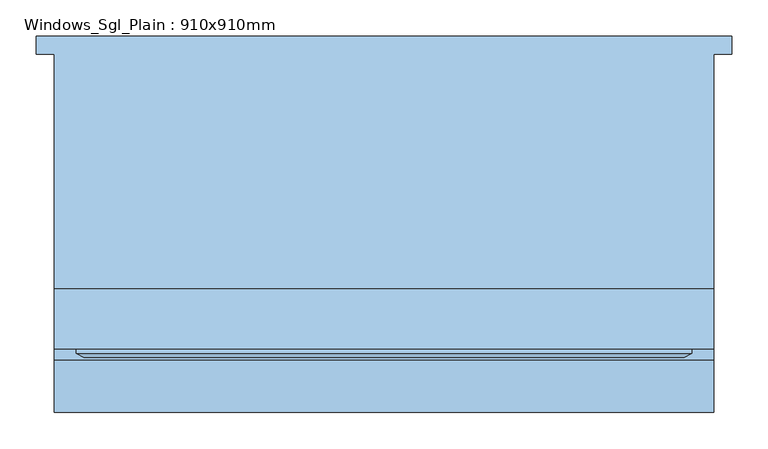
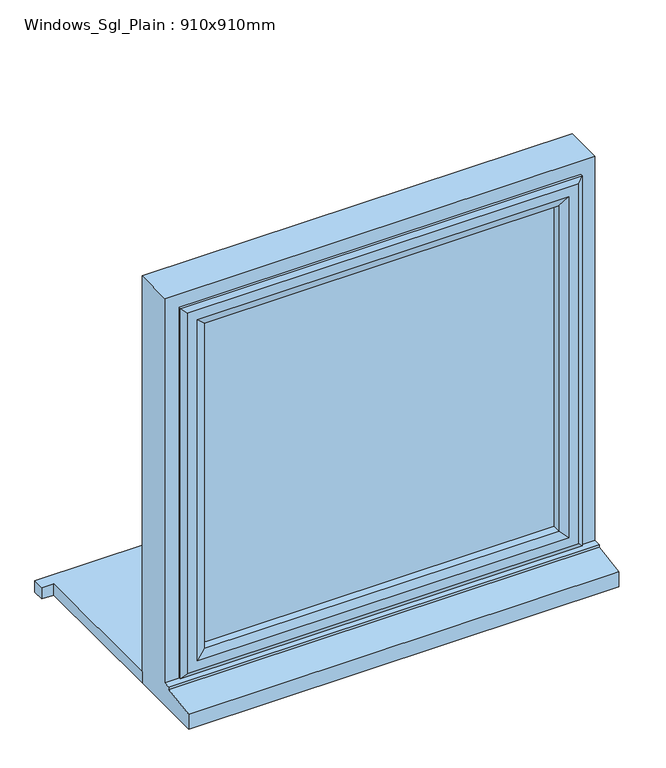
"""IFC4 building model written with IfcOpenShell, lengths in millimetres: window geometry, Windows_Sgl_Plain : 910x910mm."""

from ifc_helpers import new_model, si_unit, frame, origin, place, context, project, spatial, polyline, outline, extrude, faceted_brep, source, transform, mapped, element, save


def windows_sgl_plain_910x910mm_27dc79fa(model_context):
    return source(origin(), model_context, "Body", "SolidModel", [
        extrude(outline(polyline([(-480.0, 245.1434322), (480.0, 245.1434322), (480.0, 220.1434322), (455.0, 220.1434322), (455.0, -104.0565678), (-455.0, -104.0565678), (-455.0, 220.1434322), (-480.0, 220.1434322), (-480.0, 245.1434322)])), frame((0.0, 0.0, 1200.0), z_axis=(0.0, 0.0, 1.0), x_axis=(1.0, 0.0, 0.0)), (0.0, 0.0, 1.0), 25.0),
        faceted_brep([(-455.0, -104.0565678, 1200.0), (-455.0, -104.0565678, 2110.0), (455.0, -104.0565678, 2110.0), (455.0, -104.0565678, 1200.0), (-395.0, -104.0565678, 2050.0), (-395.0, -104.0565678, 1275.0), (395.0, -104.0565678, 1275.0), (395.0, -104.0565678, 2050.0), (-455.0, -274.5565678, 1200.0), (-455.0, -274.5565678, 1233.8088847), (-455.0, -202.0565678, 1244.7449676), (-455.0, -202.0565678, 1249.68767), (-455.0, -187.0565678, 1251.0), (-455.0, -187.0565678, 2110.0), (455.0, -187.0565678, 1251.0), (455.0, -187.0565678, 2110.0), (-415.0, -187.0565678, 2070.0), (415.0, -187.0565678, 2070.0), (415.0, -187.0565678, 1263.0), (-415.0, -187.0565678, 1263.0), (-415.0, -122.0565678, 1263.0), (-415.0, -122.0565678, 2070.0), (415.0, -122.0565678, 1263.0), (415.0, -122.0565678, 2070.0), (-395.0, -122.0565678, 2050.0), (395.0, -122.0565678, 2050.0), (395.0, -122.0565678, 1275.0), (-395.0, -122.0565678, 1275.0), (455.0, -202.0565678, 1249.68767), (455.0, -202.0565678, 1244.7449676), (455.0, -274.5565678, 1233.8088847), (455.0, -274.5565678, 1200.0)], [[[0, 1, 2, 3], [4, 5, 6, 7]], [[0, 8, 9, 10, 11, 12, 13, 1]], [[12, 14, 15, 13], [16, 17, 18, 19]], [[19, 20, 21, 16]], [[21, 20, 22, 23], [24, 25, 26, 27]], [[24, 27, 5, 4]], [[1, 13, 15, 2]], [[16, 21, 23, 17]], [[7, 25, 24, 4]], [[14, 28, 29, 30, 31, 3, 2, 15]], [[17, 23, 22, 18]], [[7, 6, 26, 25]], [[31, 8, 0, 3]], [[30, 9, 8, 31]], [[29, 10, 9, 30]], [[28, 11, 10, 29]], [[14, 12, 11, 28]], [[20, 19, 18, 22]], [[5, 27, 26, 6]]]),
        extrude(outline(polyline([(385.0, -151.0565678), (385.0, -175.0565678), (-385.0, -175.0565678), (-385.0, -151.0565678), (385.0, -151.0565678)])), frame((0.0, 0.0, 1293.0), z_axis=(0.0, 0.0, 1.0), x_axis=(1.0, 0.0, 0.0)), (0.0, 0.0, 1.0), 747.0),
        faceted_brep([(-425.0, -187.0565678, 2080.0), (-425.0, -187.0565678, 1253.0), (-425.0, -192.8300705, 1253.0), (-425.0, -192.8300705, 2080.0), (-415.0, -122.0565678, 2070.0), (-415.0, -122.0565678, 1263.0), (-415.0, -187.0565678, 1263.0), (-415.0, -187.0565678, 2070.0), (-375.0, -136.5494677, 2030.0), (-375.0, -136.5494677, 1303.0), (-385.1480377, -122.0565678, 1292.8519623), (-385.1480377, -122.0565678, 2040.1480377), (-375.0, -151.0565678, 2030.0), (-375.0, -151.0565678, 1303.0), (-385.0, -175.0565678, 2040.0), (-385.0, -175.0565678, 1293.0), (-385.0, -151.0565678, 1293.0), (-385.0, -151.0565678, 2040.0), (-375.0, -192.8300705, 2030.0), (-375.0, -192.8300705, 1303.0), (-375.0, -175.0565678, 1303.0), (-375.0, -175.0565678, 2030.0), (-392.4457548, -198.6035732, 2047.4457548), (-392.4457548, -198.6035732, 1285.5542452), (-414.2153903, -198.6035732, 1263.7846097), (-414.2153903, -198.6035732, 2069.2153903), (425.0, -187.0565678, 1253.0), (425.0, -192.8300705, 1253.0), (415.0, -122.0565678, 1263.0), (415.0, -187.0565678, 1263.0), (375.0, -136.5494677, 1303.0), (385.1480377, -122.0565678, 1292.8519623), (375.0, -151.0565678, 1303.0), (385.0, -175.0565678, 1293.0), (385.0, -151.0565678, 1293.0), (375.0, -192.8300705, 1303.0), (375.0, -175.0565678, 1303.0), (392.4457548, -198.6035732, 1285.5542452), (414.2153903, -198.6035732, 1263.7846097), (425.0, -187.0565678, 2080.0), (425.0, -192.8300705, 2080.0), (415.0, -122.0565678, 2070.0), (415.0, -187.0565678, 2070.0), (375.0, -136.5494677, 2030.0), (385.1480377, -122.0565678, 2040.1480377), (375.0, -151.0565678, 2030.0), (385.0, -175.0565678, 2040.0), (385.0, -151.0565678, 2040.0), (375.0, -192.8300705, 2030.0), (375.0, -175.0565678, 2030.0), (392.4457548, -198.6035732, 2047.4457548), (414.2153903, -198.6035732, 2069.2153903)], [[[0, 1, 2, 3]], [[4, 5, 6, 7]], [[8, 9, 10, 11]], [[12, 13, 9, 8]], [[14, 15, 16, 17]], [[18, 19, 20, 21]], [[22, 23, 19, 18]], [[3, 2, 24, 25]], [[1, 26, 27, 2]], [[5, 28, 29, 6]], [[9, 30, 31, 10]], [[13, 32, 30, 9]], [[15, 33, 34, 16]], [[19, 35, 36, 20]], [[23, 37, 35, 19]], [[2, 27, 38, 24]], [[26, 39, 40, 27]], [[28, 41, 42, 29]], [[30, 43, 44, 31]], [[32, 45, 43, 30]], [[33, 46, 47, 34]], [[35, 48, 49, 36]], [[37, 50, 48, 35]], [[27, 40, 51, 38]], [[39, 0, 3, 40]], [[1, 0, 39, 26], [7, 6, 29, 42]], [[41, 4, 7, 42]], [[5, 4, 41, 28], [11, 10, 31, 44]], [[43, 8, 11, 44]], [[45, 12, 8, 43]], [[17, 16, 34, 47], [13, 12, 45, 32]], [[46, 14, 17, 47]], [[15, 14, 46, 33], [21, 20, 36, 49]], [[48, 18, 21, 49]], [[50, 22, 18, 48]], [[25, 24, 38, 51], [23, 22, 50, 37]], [[40, 3, 25, 51]]]),
    ])


if __name__ == "__main__":
    model = new_model("IFC4")
    model_context = context("Model", 3, world=origin())
    ifc_project = project(units=[si_unit("LENGTHUNIT", "METRE", prefix="MILLI")], contexts=[model_context])
    site = spatial("IfcSite", under=ifc_project)
    building = spatial("IfcBuilding", under=site)
    placement = place(None, origin())
    windows_sgl_plain_910x910mm_shape = windows_sgl_plain_910x910mm_27dc79fa(model_context)
    element("IfcWindow", 1, ObjectType="Windows_Sgl_Plain : 910x910mm", at=placement, inside=building, context=model_context, shape_type="MappedRepresentation", body=[
        mapped(windows_sgl_plain_910x910mm_shape, transform((0.0, 0.0, 0.0), x_axis=(1.0, 0.0, 0.0), y_axis=(0.0, 1.0, 0.0), z_axis=(0.0, 0.0, 1.0))),
    ])
    save(model, "model.ifc")

# Revit data of these elements
# Type "Windows_Sgl_Plain : 910x910mm"
#   Type Mark = "44"
#   Operation = "SinglePanel"
#   Construction Type Id = "SGL"
#   Manufacturer = "Revit"
#   Keynote = "L10"
#   Analytic Construction = "Large single-glazed windows"
#   Wrap Layers (Ext) from Ext = 102.5 mm
#   Wrap Layers (Int) from Ext = 177.5 mm
#   Window Board Projection = 25 mm
#   Window Board Extension = 25 mm
#   Visual Light Transmittance = 0.9
#   Solar Heat Gain Coefficient = 0.86
#   Rough Width = 910 mm
#   Rough Height = 910 mm
#   Height = 910 mm
#   Width = 910 mm
#   Heat Transfer Coefficient (U) = 5.5617 W/(m²·K)
#   Glazing Thickness = 24 mm
#   FrameOffset - External = 50 mm
#   Frame Depth = 65 mm
#   Default Head Height = 2110 mm
#   Cill Depth = 87.5 mm
#   Cavity Closer Width = 50 mm
#   Cavity Closer Offset from Ext = 102.5 mm
#   Cavity Closer Depth = 85 mm
#   Define Thermal Properties by = 1
#   Vis - Cavity Closers = yes
#   Define Thermal Properties by = 1
#   Material Trim = Window Frame
#   Material Glass = Glass
#   Material Frame = Window Frame
#   Wall Closure = (empty or 0)
# Element 1 (IfcWindow, "Windows_Sgl_Plain : 910x910mm")
#   Materials on its faces: "Window Frame", "Glass"
# Materials
#   "Window Frame": colour RGB 249 249 249, transparency 0, Keynote = "L10", Cost = 0
#   "Glass": class "Glass", colour RGB 0 128 192, transparency 0.9, Description = "Soda Lime Glass", Cost = 0
